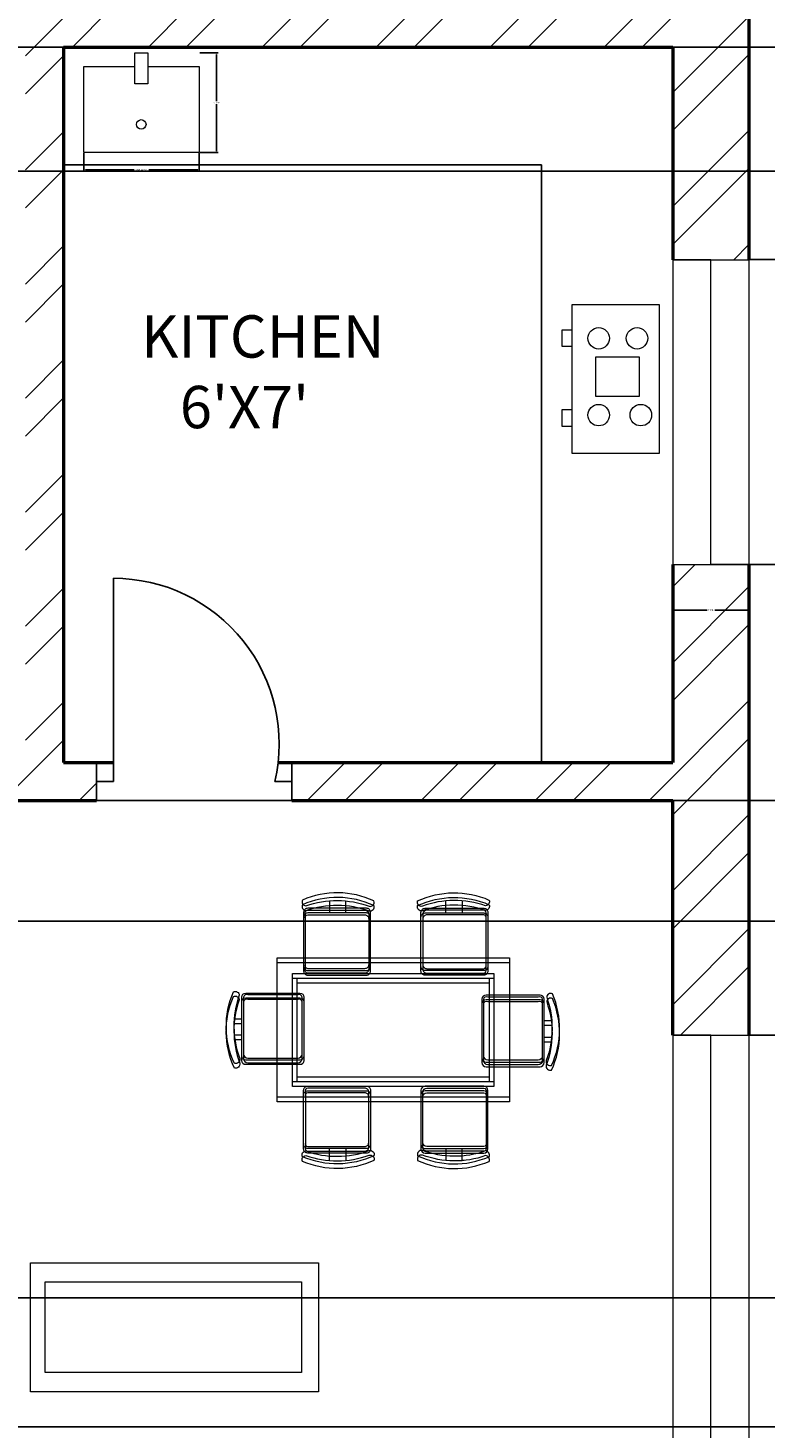
# Model space of a CAD drawing. Units: inches. Extents: x 2310 to 2937, y 1113 to 2410.
# Tile 21 of 23: x 2739 to 2826, y 2132 to 2297. Entities that reach past the tile are written whole.
import ezdxf

# ---------------------------------------------------------------- set-up
doc = ezdxf.new("R2010")
doc.units = ezdxf.units.IN
for name, color, linetype, lineweight in [('A-ANNO-DIMS', 2, 'Continuous', 18), ('A-AREA-IDEN', 7, 'Continuous', 18), ('A-DOOR', 31, 'Continuous', 25), ('A-EQPM', 8, 'Continuous', 18), ('A-FLOR-CASE', 7, 'Continuous', 25), ('A-FLOR-FIXT', 9, 'Continuous', 18), ('A-FURN', 8, 'Continuous', 18), ('A-GLAZ', 191, 'Continuous', 20), ('A-WALL', 7, 'Continuous', 50), ('A-WALL-PATT', 85, 'Continuous', 13)]:
    doc.layers.add(name, color=color, linetype=linetype, lineweight=lineweight)
doc.styles.get("Standard").update_dxf_attribs({"font": 'arial.ttf'})
doc.dimstyles.get("Standard").update_dxf_attribs({"dimtxt": 0.18, "dimasz": 0.18, "dimexe": 0.18, "dimexo": 0.0625, "dimgap": 0.09, "dimtad": 0, "dimtih": 1, "dimtoh": 1, "dimdec": 4, "dimzin": 0, "dimdsep": 46, "dimtxsty": 'Standard', "dimcen": 0.09, "dimadec": 0, "dimazin": 0, "dimtfac": 1, "dimtdec": 4, "dimtofl": 0, "dimtmove": 0, "dimatfit": 3, "dimfxl": 1, "dimtolj": 1, "dimtzin": 0, "dimarcsym": 0})

# ---------------------------------------------------------------- blocks, each defined once
blk = doc.blocks.new('SINK-KITCHEN')
blk.add_lwpolyline([(6.01, 11.79), (7.56, 11.79), (7.56, 8.11), (6.01, 8.11)], close=True)
blk.add_lwpolyline([(7.56, 10.17), (13.64, 10.17), (13.64, 0), (0, 0), (0, 10.17), (6.01, 10.17)])
blk.add_circle((6.79, 3.34), 0.556)
blk = doc.blocks.new('RANGE-4-BURNER')
for points in [[(1.2, 17.61), (1.2, 17.61), (1.2, 17.61), (1.2, 17.61)], [(1.2, 17.61), (11.5, 17.61), (11.5, 0), (1.2, 0)], [(1.2, 14.58), (0, 14.58), (0, 12.67), (1.2, 12.67)], [(4.01, 11.43), (9.13, 11.43), (9.13, 6.73), (4.01, 6.73)], [(1.2, 5.14), (0, 5.14), (0, 3.24), (1.2, 3.24)]]:
    blk.add_lwpolyline(points, close=True)
for centre in [(4.34, 13.6), (8.87, 13.6), (4.34, 4.53), (9.32, 4.53)]:
    blk.add_circle(centre, 1.27)
blk = doc.blocks.new('WIN-36IN')
for p, q in [((4.5, 36), (0, 36)), ((0, 36), (9, 36)), ((0, 36), (0, 0)), ((4.5, 0), (4.5, 36)), ((9, 36), (9, 0)), ((0, 0), (9, 0)), ((9, 0), (4.5, 0))]:
    blk.add_line(p, q)
blk = doc.blocks.new('DINING-TABLE')
for points in [[(0, 17.02), (27.45, 17.02), (27.45, 0.55), (0, 0.55)], [(0, 17.02), (27.45, 17.02), (27.45, 0.55), (0, 0.55)], [(0, 16.47), (27.45, 16.47), (27.45, 0), (0, 0)], [(0, 16.47), (27.45, 16.47), (27.45, 0), (0, 0)], [(1.83, 15.19), (25.62, 15.19), (25.62, 2.38), (1.83, 2.38)], [(1.83, 15.19), (25.62, 15.19), (25.62, 2.38), (1.83, 2.38)], [(1.83, 14.64), (25.62, 14.64), (25.62, 1.83), (1.83, 1.83)], [(1.83, 14.64), (25.62, 14.64), (25.62, 1.83), (1.83, 1.83)], [(2.38, 14.64), (25.07, 14.64), (25.07, 2.93), (2.38, 2.93)], [(2.38, 14.64), (25.07, 14.64), (25.07, 2.93), (2.38, 2.93)], [(2.38, 14.09), (25.07, 14.09), (25.07, 2.38), (2.38, 2.38)], [(2.38, 14.09), (25.07, 14.09), (25.07, 2.38), (2.38, 2.38)]]:
    blk.add_lwpolyline(points, close=True)
blk = doc.blocks.new('CHAIR-DINING')
for points in [[(0.62, 8.14, -0.578392), (0.05, 8.77, -0.214524), (8.49, 8.88, -0.552014), (8.09, 8.2, 0.175809), (0.62, 8.14)], [(0.62, 8.14, -0.578392), (0.05, 8.77, -0.214524), (8.49, 8.88, -0.552014), (8.09, 8.2, 0.175809), (0.62, 8.14)], [(0.62, 7.6, -0.578392), (0.05, 8.22, -0.214524), (8.49, 8.33, -0.552014), (8.09, 7.65, 0.175809), (0.62, 7.6)], [(0.62, 7.6, -0.578392), (0.05, 8.22, -0.214524), (8.49, 8.33, -0.552014), (8.09, 7.65, 0.175809), (0.62, 7.6)], [(3.37, 7.9), (3.37, 8.78, 0.064759)], [(3.37, 7.9), (3.37, 8.78, 0.064759)], [(7.88, 7.9, -0.414214), (8.36, 7.42), (8.36, 1.03, -0.414214), (7.88, 0.55), (0.94, 0.55, -0.414214), (0.45, 1.03), (0.45, 7.42, -0.414214), (0.94, 7.9), (7.88, 7.9)], [(7.88, 7.9, -0.414214), (8.36, 7.42), (8.36, 1.03, -0.414214), (7.88, 0.55), (0.94, 0.55, -0.414214), (0.45, 1.03), (0.45, 7.42, -0.414214), (0.94, 7.9), (7.88, 7.9)], [(7.88, 7.35, -0.414214), (8.36, 6.87), (8.36, 0.49, -0.414214), (7.88, 0), (0.94, 0, -0.414214), (0.45, 0.49), (0.45, 6.87, -0.414214), (0.94, 7.35), (7.88, 7.35)], [(7.88, 7.35, -0.414214), (8.36, 6.87), (8.36, 0.49, -0.414214), (7.88, 0), (0.94, 0, -0.414214), (0.45, 0.49), (0.45, 6.87, -0.414214), (0.94, 7.35), (7.88, 7.35)], [(3.37, 7.35), (3.37, 8.23, 0.064759)], [(3.37, 7.35), (3.37, 8.23, 0.064759)]]:
    blk.add_lwpolyline(points, format="xyb")
for points in [[(5.32, 8.8), (5.32, 7.9)], [(5.32, 8.79), (5.32, 7.9)], [(5.32, 8.25), (5.32, 7.35)], [(5.32, 8.25), (5.32, 7.35)]]:
    blk.add_lwpolyline(points)
for points in [[(7.87, 7.68), (1.16, 7.68, 0.414214), (0.67, 7.2), (0.67, 1.25, 0.414214), (1.16, 0.77), (7.87, 0.77, 0.512069), (8.14, 1.25), (8.14, 7.2, 0.512069)], [(7.87, 7.68), (1.16, 7.68, 0.414214), (0.67, 7.2), (0.67, 1.25, 0.414214), (1.16, 0.77), (7.87, 0.77, 0.512069), (8.14, 1.25), (8.14, 7.2, 0.512069)], [(7.87, 7.13), (1.16, 7.13, 0.414214), (0.67, 6.65), (0.67, 0.7, 0.414214), (1.16, 0.22), (7.87, 0.22, 0.512069), (8.14, 0.7), (8.14, 6.65, 0.512069)], [(7.87, 7.13), (1.16, 7.13, 0.414214), (0.67, 6.65), (0.67, 0.7, 0.414214), (1.16, 0.22), (7.87, 0.22, 0.512069), (8.14, 0.7), (8.14, 6.65, 0.512069)]]:
    blk.add_lwpolyline(points, format="xyb", close=True)
blk = doc.blocks.new('CHAIR-DINING-3')
for points in [[(0.47, 8.2, -0.175809), (7.95, 8.14, 0.578392), (8.51, 8.77, 0.214524), (0.07, 8.88, 0.552014), (0.47, 8.2, -0.065079)], [(0.47, 8.2, -0.175809), (7.95, 8.14, 0.578392), (8.51, 8.77, 0.214524), (0.07, 8.88, 0.552014), (0.47, 8.2, -0.065079)], [(0.47, 7.65, -0.175809), (7.95, 7.6, 0.578392), (8.51, 8.22, 0.214524), (0.07, 8.33, 0.552014), (0.47, 7.65, -0.065079)], [(0.47, 7.65, -0.175809), (7.95, 7.6, 0.578392), (8.51, 8.22, 0.214524), (0.07, 8.33, 0.552014), (0.47, 7.65, -0.065079)], [(5.19, 7.9), (5.19, 8.78, -0.064759)], [(5.19, 7.9), (5.19, 8.78, -0.064759)], [(7.63, 7.9), (0.69, 7.9, 0.414214), (0.2, 7.42), (0.2, 1.03, 0.414214), (0.69, 0.55), (7.63, 0.55, 0.414214), (8.11, 1.03), (8.11, 7.42, 0.414214), (7.63, 7.9)], [(7.63, 7.9), (0.69, 7.9, 0.414214), (0.2, 7.42), (0.2, 1.03, 0.414214), (0.69, 0.55), (7.63, 0.55, 0.414214), (8.11, 1.03), (8.11, 7.42, 0.414214), (7.63, 7.9)], [(7.63, 7.35), (0.69, 7.35, 0.414214), (0.2, 6.87), (0.2, 0.49, 0.414214), (0.69, 0), (7.63, 0, 0.414214), (8.11, 0.49), (8.11, 6.87, 0.414214), (7.63, 7.35)], [(7.63, 7.35), (0.69, 7.35, 0.414214), (0.2, 6.87), (0.2, 0.49, 0.414214), (0.69, 0), (7.63, 0, 0.414214), (8.11, 0.49), (8.11, 6.87, 0.414214), (7.63, 7.35)], [(5.19, 7.35), (5.19, 8.23, -0.064759)], [(5.19, 7.35), (5.19, 8.23, -0.064759)]]:
    blk.add_lwpolyline(points, format="xyb")
for points in [[(3.25, 8.8), (3.25, 7.9)], [(3.25, 8.79), (3.25, 7.9)], [(3.25, 8.25), (3.25, 7.35)], [(3.25, 8.25), (3.25, 7.35)]]:
    blk.add_lwpolyline(points)
for points in [[(0.69, 7.68), (7.41, 7.68, -0.414214), (7.9, 7.2), (7.9, 1.25, -0.414214), (7.41, 0.77), (0.69, 0.77, -0.512069), (0.42, 1.25), (0.42, 7.2, -0.512069)], [(0.69, 7.68), (7.41, 7.68, -0.414214), (7.9, 7.2), (7.9, 1.25, -0.414214), (7.41, 0.77), (0.69, 0.77, -0.512069), (0.42, 1.25), (0.42, 7.2, -0.512069)], [(0.69, 7.13), (7.41, 7.13, -0.414214), (7.9, 6.65), (7.9, 0.7, -0.414214), (7.41, 0.22), (0.69, 0.22, -0.512069), (0.42, 0.7), (0.42, 6.65, -0.512069)], [(0.69, 7.13), (7.41, 7.13, -0.414214), (7.9, 6.65), (7.9, 0.7, -0.414214), (7.41, 0.22), (0.69, 0.22, -0.512069), (0.42, 0.7), (0.42, 6.65, -0.512069)]]:
    blk.add_lwpolyline(points, format="xyb", close=True)
blk = doc.blocks.new('CHAIR-DINING-4')
for points in [[(0.62, 8.14, -0.578392), (0.05, 8.77, -0.214524), (8.49, 8.88, -0.552014), (8.09, 8.2, 0.175809), (0.62, 8.14)], [(0.62, 8.14, -0.578392), (0.05, 8.77, -0.214524), (8.49, 8.88, -0.552014), (8.09, 8.2, 0.175809), (0.62, 8.14)], [(0.62, 7.6, -0.578392), (0.05, 8.22, -0.214524), (8.49, 8.33, -0.552014), (8.09, 7.65, 0.175809), (0.62, 7.6)], [(0.62, 7.6, -0.578392), (0.05, 8.22, -0.214524), (8.49, 8.33, -0.552014), (8.09, 7.65, 0.175809), (0.62, 7.6)], [(3.37, 7.9), (3.37, 8.78, 0.064759)], [(3.37, 7.9), (3.37, 8.78, 0.064759)], [(7.88, 7.9, -0.414214), (8.36, 7.42), (8.36, 1.03, -0.414214), (7.88, 0.55), (0.94, 0.55, -0.414214), (0.45, 1.03), (0.45, 7.42, -0.414214), (0.94, 7.9), (7.88, 7.9)], [(7.88, 7.9, -0.414214), (8.36, 7.42), (8.36, 1.03, -0.414214), (7.88, 0.55), (0.94, 0.55, -0.414214), (0.45, 1.03), (0.45, 7.42, -0.414214), (0.94, 7.9), (7.88, 7.9)], [(7.88, 7.35, -0.414214), (8.36, 6.87), (8.36, 0.49, -0.414214), (7.88, 0), (0.94, 0, -0.414214), (0.45, 0.49), (0.45, 6.87, -0.414214), (0.94, 7.35), (7.88, 7.35)], [(7.88, 7.35, -0.414214), (8.36, 6.87), (8.36, 0.49, -0.414214), (7.88, 0), (0.94, 0, -0.414214), (0.45, 0.49), (0.45, 6.87, -0.414214), (0.94, 7.35), (7.88, 7.35)], [(3.37, 7.35), (3.37, 8.23, 0.064759)], [(3.37, 7.35), (3.37, 8.23, 0.064759)]]:
    blk.add_lwpolyline(points, format="xyb")
for points in [[(5.32, 8.8), (5.32, 7.9)], [(5.32, 8.79), (5.32, 7.9)], [(5.32, 8.25), (5.32, 7.35)], [(5.32, 8.25), (5.32, 7.35)]]:
    blk.add_lwpolyline(points)
for points in [[(7.87, 7.68), (1.16, 7.68, 0.414214), (0.67, 7.2), (0.67, 1.25, 0.414214), (1.16, 0.77), (7.87, 0.77, 0.512069), (8.14, 1.25), (8.14, 7.2, 0.512069)], [(7.87, 7.68), (1.16, 7.68, 0.414214), (0.67, 7.2), (0.67, 1.25, 0.414214), (1.16, 0.77), (7.87, 0.77, 0.512069), (8.14, 1.25), (8.14, 7.2, 0.512069)], [(7.87, 7.13), (1.16, 7.13, 0.414214), (0.67, 6.65), (0.67, 0.7, 0.414214), (1.16, 0.22), (7.87, 0.22, 0.512069), (8.14, 0.7), (8.14, 6.65, 0.512069)], [(7.87, 7.13), (1.16, 7.13, 0.414214), (0.67, 6.65), (0.67, 0.7, 0.414214), (1.16, 0.22), (7.87, 0.22, 0.512069), (8.14, 0.7), (8.14, 6.65, 0.512069)]]:
    blk.add_lwpolyline(points, format="xyb", close=True)
blk = doc.blocks.new('*D23')
at = {"layer": 'A-ANNO-DIMS', "color": 0, "lineweight": -2, "transparency": 16777216}
for p, q in [((2745.39, 2282.48), (2745.39, 2280.32)), ((2759.02, 2282.48), (2759.02, 2280.32)), ((2745.57, 2280.5), (2751.35, 2280.5)), ((2758.84, 2280.5), (2753.06, 2280.5))]:
    blk.add_line(p, q, dxfattribs=at)
at = {"layer": 'A-ANNO-DIMS', "color": 0, "transparency": 16777216}
for points in [[(2745.57, 2280.53), (2745.57, 2280.47), (2745.39, 2280.5)], [(2758.84, 2280.53), (2758.84, 2280.47), (2759.02, 2280.5)]]:
    blk.add_solid(points, dxfattribs=at)
at = {"layer": 'Defpoints', "color": 0, "transparency": 16777216}
for p in [(2745.39, 2282.54), (2759.02, 2282.54), (2759.02, 2280.5)]:
    blk.add_point(p, dxfattribs=at)
at = {"layer": 'A-ANNO-DIMS', "color": 0, "transparency": 16777216, "insert": (2752.2, 2280.5), "char_height": 0.18, "attachment_point": 5}
blk.add_mtext('\\A1;SINK 14 TYP.', dxfattribs=at)
blk = doc.blocks.new('*D24')
at = {"layer": 'A-ANNO-DIMS', "color": 0, "lineweight": -2, "transparency": 16777216}
for p, q in [((2759.09, 2294.33), (2761.25, 2294.33)), ((2761.07, 2294.15), (2761.07, 2288.62)), ((2761.07, 2282.72), (2761.07, 2288.26)), ((2759.09, 2282.54), (2761.25, 2282.54))]:
    blk.add_line(p, q, dxfattribs=at)
at = {"layer": 'A-ANNO-DIMS', "color": 0, "transparency": 16777216}
for points in [[(2761.04, 2294.15), (2761.1, 2294.15), (2761.07, 2294.33)], [(2761.04, 2282.72), (2761.1, 2282.72), (2761.07, 2282.54)]]:
    blk.add_solid(points, dxfattribs=at)
at = {"layer": 'Defpoints', "color": 0, "transparency": 16777216}
for p in [(2759.02, 2294.33), (2761.07, 2294.33), (2759.02, 2282.54)]:
    blk.add_point(p, dxfattribs=at)
at = {"layer": 'A-ANNO-DIMS', "color": 0, "transparency": 16777216, "insert": (2761.07, 2288.44), "char_height": 0.18, "attachment_point": 5}
blk.add_mtext('\\A1;12 TYP.', dxfattribs=at)
blk = doc.blocks.new('*D31')
at = {"layer": 'A-ANNO-DIMS', "color": 0, "lineweight": -2, "transparency": 16777216}
for p, q in [((2824.05, 2269.9), (2829.57, 2269.9)), ((2829.39, 2269.72), (2829.39, 2252.08)), ((2829.39, 2234.08), (2829.39, 2251.71)), ((2824.05, 2233.9), (2829.57, 2233.9))]:
    blk.add_line(p, q, dxfattribs=at)
at = {"layer": 'A-ANNO-DIMS', "color": 0, "transparency": 16777216}
for points in [[(2829.36, 2269.72), (2829.42, 2269.72), (2829.39, 2269.9)], [(2829.36, 2234.08), (2829.42, 2234.08), (2829.39, 2233.9)]]:
    blk.add_solid(points, dxfattribs=at)
at = {"layer": 'Defpoints', "color": 0, "transparency": 16777216}
for p in [(2823.99, 2269.9), (2829.39, 2269.9), (2823.99, 2233.9)]:
    blk.add_point(p, dxfattribs=at)
at = {"layer": 'A-ANNO-DIMS', "color": 0, "transparency": 16777216, "insert": (2829.39, 2251.9), "char_height": 0.18, "attachment_point": 5}
blk.add_mtext('\\A1;WINDOW 36 TYP.', dxfattribs=at)
blk = doc.blocks.new('*D32')
at = {"layer": 'A-ANNO-DIMS', "color": 0, "lineweight": -2, "transparency": 16777216}
for p, q in [((2814.99, 2233.84), (2814.99, 2228.32)), ((2823.99, 2233.84), (2823.99, 2228.32)), ((2815.17, 2228.5), (2819.03, 2228.5)), ((2823.81, 2228.5), (2819.94, 2228.5))]:
    blk.add_line(p, q, dxfattribs=at)
at = {"layer": 'A-ANNO-DIMS', "color": 0, "transparency": 16777216}
for points in [[(2815.17, 2228.53), (2815.17, 2228.47), (2814.99, 2228.5)], [(2823.81, 2228.53), (2823.81, 2228.47), (2823.99, 2228.5)]]:
    blk.add_solid(points, dxfattribs=at)
at = {"layer": 'Defpoints', "color": 0, "transparency": 16777216}
for p in [(2814.99, 2233.9), (2823.99, 2233.9), (2823.99, 2228.5)]:
    blk.add_point(p, dxfattribs=at)
at = {"layer": 'A-ANNO-DIMS', "color": 0, "transparency": 16777216, "insert": (2819.49, 2228.5), "char_height": 0.18, "attachment_point": 5}
blk.add_mtext('\\A1;9 TYP.', dxfattribs=at)
blk = doc.blocks.new('*D49')
at = {"layer": 'A-ANNO-DIMS', "color": 0, "lineweight": -2, "transparency": 16777216}
for p, q in [((2824.05, 2233.9), (2858.02, 2233.9)), ((2857.84, 2233.72), (2857.84, 2206.28)), ((2857.84, 2178.48), (2857.84, 2205.92)), ((2824.05, 2178.3), (2858.02, 2178.3))]:
    blk.add_line(p, q, dxfattribs=at)
at = {"layer": 'A-ANNO-DIMS', "color": 0, "transparency": 16777216}
for points in [[(2857.81, 2233.72), (2857.87, 2233.72), (2857.84, 2233.9)], [(2857.81, 2178.48), (2857.87, 2178.48), (2857.84, 2178.3)]]:
    blk.add_solid(points, dxfattribs=at)
at = {"layer": 'Defpoints', "color": 0, "transparency": 16777216}
for p in [(2823.99, 2233.9), (2857.84, 2233.9), (2823.99, 2178.3)]:
    blk.add_point(p, dxfattribs=at)
at = {"layer": 'A-ANNO-DIMS', "color": 0, "transparency": 16777216, "insert": (2857.84, 2206.1), "char_height": 0.18, "attachment_point": 5}
blk.add_mtext('\\A1;55.6', dxfattribs=at)
blk = doc.blocks.new('*D50')
at = {"layer": 'A-ANNO-DIMS', "color": 0, "lineweight": -2, "transparency": 16777216}
for p, q in [((2824.05, 2312.76), (2858.02, 2312.76)), ((2857.84, 2312.58), (2857.84, 2291.51)), ((2857.84, 2270.08), (2857.84, 2291.15)), ((2824.05, 2269.9), (2858.02, 2269.9))]:
    blk.add_line(p, q, dxfattribs=at)
at = {"layer": 'A-ANNO-DIMS', "color": 0, "transparency": 16777216}
for points in [[(2857.81, 2312.58), (2857.87, 2312.58), (2857.84, 2312.76)], [(2857.81, 2270.08), (2857.87, 2270.08), (2857.84, 2269.9)]]:
    blk.add_solid(points, dxfattribs=at)
at = {"layer": 'Defpoints', "color": 0, "transparency": 16777216}
for p in [(2823.99, 2312.76), (2857.84, 2312.76), (2823.99, 2269.9)]:
    blk.add_point(p, dxfattribs=at)
at = {"layer": 'A-ANNO-DIMS', "color": 0, "transparency": 16777216, "insert": (2857.84, 2291.33), "char_height": 0.18, "attachment_point": 5}
blk.add_mtext('\\A1;42.86', dxfattribs=at)
blk = doc.blocks.new('*D53')
at = {"layer": 'A-ANNO-DIMS', "color": 0, "lineweight": -2, "transparency": 16777216}
for p, q in [((2403.55, 2295.01), (2858.02, 2295.01)), ((2857.84, 2294.83), (2857.84, 2287.87)), ((2857.84, 2280.55), (2857.84, 2287.51)), ((2403.55, 2280.37), (2858.02, 2280.37))]:
    blk.add_line(p, q, dxfattribs=at)
at = {"layer": 'A-ANNO-DIMS', "color": 0, "transparency": 16777216}
for points in [[(2857.81, 2294.83), (2857.87, 2294.83), (2857.84, 2295.01)], [(2857.81, 2280.55), (2857.87, 2280.55), (2857.84, 2280.37)]]:
    blk.add_solid(points, dxfattribs=at)
at = {"layer": 'Defpoints', "color": 0, "transparency": 16777216}
for p in [(2403.49, 2295.01), (2403.49, 2280.37), (2857.84, 2280.37)]:
    blk.add_point(p, dxfattribs=at)
at = {"layer": 'A-ANNO-DIMS', "color": 0, "transparency": 16777216, "insert": (2857.84, 2287.69), "char_height": 0.18, "attachment_point": 5}
blk.add_mtext('\\A1;14.644', dxfattribs=at)
blk = doc.blocks.new('*D54')
at = {"layer": 'A-ANNO-DIMS', "color": 0, "lineweight": -2, "transparency": 16777216}
for p, q in [((2403.55, 2206.01), (2858.02, 2206.01)), ((2857.84, 2205.83), (2857.84, 2199.07)), ((2857.84, 2191.94), (2857.84, 2198.7)), ((2403.55, 2191.76), (2858.02, 2191.76))]:
    blk.add_line(p, q, dxfattribs=at)
at = {"layer": 'A-ANNO-DIMS', "color": 0, "transparency": 16777216}
for points in [[(2857.81, 2205.83), (2857.87, 2205.83), (2857.84, 2206.01)], [(2857.81, 2191.94), (2857.87, 2191.94), (2857.84, 2191.76)]]:
    blk.add_solid(points, dxfattribs=at)
at = {"layer": 'Defpoints', "color": 0, "transparency": 16777216}
for p in [(2403.49, 2206.01), (2403.49, 2191.76), (2857.84, 2191.76)]:
    blk.add_point(p, dxfattribs=at)
at = {"layer": 'A-ANNO-DIMS', "color": 0, "transparency": 16777216, "insert": (2857.84, 2198.89), "char_height": 0.18, "attachment_point": 5}
blk.add_mtext('\\A1;14.255', dxfattribs=at)
blk = doc.blocks.new('*D70')
at = {"layer": 'A-ANNO-DIMS', "color": 0, "lineweight": -2, "transparency": 16777216}
for p, q in [((2475.96, 2147.28), (2858.02, 2147.28)), ((2857.84, 2147.1), (2857.84, 2139.83)), ((2857.84, 2132.2), (2857.84, 2139.47)), ((2475.96, 2132.02), (2858.02, 2132.02))]:
    blk.add_line(p, q, dxfattribs=at)
at = {"layer": 'A-ANNO-DIMS', "color": 0, "transparency": 16777216}
for points in [[(2857.81, 2147.1), (2857.87, 2147.1), (2857.84, 2147.28)], [(2857.81, 2132.2), (2857.87, 2132.2), (2857.84, 2132.02)]]:
    blk.add_solid(points, dxfattribs=at)
at = {"layer": 'Defpoints', "color": 0, "transparency": 16777216}
for p in [(2475.89, 2147.28), (2857.84, 2147.28), (2475.89, 2132.02)]:
    blk.add_point(p, dxfattribs=at)
at = {"layer": 'A-ANNO-DIMS', "color": 0, "transparency": 16777216, "insert": (2857.84, 2139.65), "char_height": 0.18, "attachment_point": 5}
blk.add_mtext('\\A1;15.257', dxfattribs=at)

msp = doc.modelspace()

# ---------------------------------------------------------------- hatches: boundary and pattern name
at = {"layer": 'A-WALL-PATT'}
h = msp.add_hatch(dxfattribs=at)
h.set_pattern_fill('ANSI32', color=256)
h.paths.add_polyline_path([(2639.1394, 2356.5139), (2563.662, 2356.5139), (2563.662, 2347.5139), (2606.9859, 2347.5139), (2606.9859, 2210.5139), (2514.2692, 2210.5139), (2514.2692, 2206.0139), (2606.9859, 2206.0139), (2606.9859, 2098.0139), (2602.689, 2098.0139), (2602.689, 2093.5139), (2615.5262, 2093.5139), (2615.5262, 2095.7639), (2615.5262, 2098.0139), (2611.4859, 2098.0139), (2611.4859, 2206.0139), (2703.9391, 2206.0139), (2703.9391, 2208.2639), (2703.9391, 2210.5139), (2611.4859, 2210.5139), (2611.4859, 2347.5139), (2639.1394, 2347.5139)])
h.paths.add_polyline_path([(2823.9859, 2356.5139), (2699.1394, 2356.5139), (2699.1394, 2347.5139), (2738.4859, 2347.5139), (2738.4859, 2343.9266), (2742.9859, 2343.9266), (2742.9859, 2347.5139), (2814.9859, 2347.5139), (2814.9859, 2336.76), (2823.9859, 2336.76)])
h.paths.add_polyline_path([(2823.9859, 2312.76), (2814.9859, 2312.76), (2814.9859, 2299.5139), (2742.9859, 2299.5139), (2742.9859, 2323.0159), (2740.7359, 2323.0159), (2738.4859, 2323.0159), (2738.4859, 2210.5139), (2734.5483, 2210.5139), (2734.5483, 2206.0139), (2746.8769, 2206.0139), (2746.8769, 2208.2639), (2746.8769, 2210.5139), (2742.9859, 2210.5139), (2742.9859, 2295.0139), (2814.9859, 2295.0139), (2814.9859, 2269.8977), (2823.9859, 2269.8977)])
h.paths.add_polyline_path([(2823.9859, 2210.5139), (2823.9859, 2233.8977), (2819.4859, 2233.8977), (2814.9859, 2233.8977), (2814.9859, 2210.5139), (2769.9745, 2210.5139), (2769.9745, 2206.0139), (2814.9859, 2206.0139), (2814.9859, 2178.3027), (2823.9859, 2178.3027)])
h.paths.add_polyline_path([(2823.9859, 2118.3027), (2819.4859, 2118.3027), (2814.9859, 2118.3027), (2814.9859, 2098.0139), (2647.0333, 2098.0139), (2647.0333, 2093.5139), (2814.9859, 2093.5139), (2814.9859, 1999.5139), (2650.6052, 1999.5139), (2650.6052, 1995.0139), (2814.9859, 1995.0139), (2814.9859, 1969.9784), (2823.9859, 1969.9784)])
h.paths.add_polyline_path([(2403.4859, 2093.5139), (2569.9888, 2093.5139), (2569.9888, 2095.7639), (2569.9888, 2098.0139), (2403.4859, 2098.0139), (2403.4859, 2131.7587), (2394.4859, 2131.7587), (2394.4859, 1967.522), (2403.4859, 1967.522), (2403.4859, 1995.0139), (2569.8903, 1995.0139), (2569.8903, 1997.2639), (2569.8903, 1999.5139), (2403.4859, 1999.5139)])
h.paths.add_polyline_path([(2503.662, 2356.5139), (2394.4859, 2356.5139), (2394.4859, 2337.9231), (2398.9859, 2337.9231), (2403.4859, 2337.9231), (2403.4859, 2347.5139), (2475.4859, 2347.5139), (2475.4859, 2343.0384), (2479.9859, 2343.0384), (2479.9859, 2347.5139), (2503.662, 2347.5139)])
h.paths.add_polyline_path([(2498.3065, 1745.5139), (2479.9859, 1745.5139), (2479.9859, 1749.1663), (2477.7359, 1749.1663), (2475.4859, 1749.1663), (2475.4859, 1745.5139), (2403.4859, 1745.5139), (2403.4859, 1753.6409), (2398.9859, 1753.6409), (2394.4859, 1753.6409), (2394.4859, 1736.5139), (2498.3065, 1736.5139), (2498.3065, 1741.0139)])
h.paths.add_polyline_path([(2479.9859, 1882.5139), (2483.9367, 1882.5139), (2483.9367, 1887.0139), (2471.5501, 1887.0139), (2471.5501, 1885.1969), (2471.5501, 1882.5139), (2475.4859, 1882.5139), (2475.4859, 1798.0139), (2403.4859, 1798.0139), (2403.4859, 1828.0433), (2402.2852, 1828.0433), (2394.4859, 1828.0433), (2394.4859, 1777.6409), (2403.4859, 1777.6409), (2403.4859, 1793.5139), (2475.4859, 1793.5139), (2475.4859, 1769.1696), (2479.9859, 1769.1696)])
h.paths.add_polyline_path([(2403.4859, 1907.522), (2398.9859, 1907.522), (2394.4859, 1907.522), (2394.4859, 1864.0433), (2403.4859, 1864.0433), (2403.4859, 1882.5139), (2448.9325, 1882.5139), (2448.9325, 1884.7639), (2448.9325, 1887.0139), (2403.4859, 1887.0139)])
h.paths.add_polyline_path([(2702.2061, 1887.0139), (2611.4859, 1887.0139), (2611.4859, 1995.0139), (2615.6132, 1995.0139), (2615.6132, 1999.5139), (2602.4798, 1999.5139), (2602.4798, 1997.2639), (2602.4798, 1995.0139), (2606.9859, 1995.0139), (2606.9859, 1887.0139), (2516.2443, 1887.0139), (2516.2443, 1884.7639), (2516.2443, 1882.5139), (2606.9859, 1882.5139), (2606.9859, 1745.5139), (2558.3065, 1745.5139), (2558.3065, 1736.5139), (2638.8921, 1736.5139), (2638.8921, 1741.0139), (2638.8921, 1745.5139), (2611.4859, 1745.5139), (2611.4859, 1882.5139), (2702.2061, 1882.5139)])
h.paths.add_polyline_path([(2823.9859, 1909.9784), (2819.4859, 1909.9784), (2814.9859, 1909.9784), (2814.9859, 1887.0139), (2769.144, 1887.0139), (2769.144, 1884.7639), (2769.144, 1882.5139), (2814.9859, 1882.5139), (2814.9859, 1854.1704), (2823.9859, 1854.1704)])
h.paths.add_polyline_path([(2823.9859, 1818.1704), (2819.4859, 1818.1704), (2814.9859, 1818.1704), (2814.9859, 1798.0139), (2742.9859, 1798.0139), (2742.9859, 1882.5139), (2746.805, 1882.5139), (2746.805, 1887.0139), (2733.7334, 1887.0139), (2733.7334, 1884.7639), (2733.7334, 1882.5139), (2738.4859, 1882.5139), (2738.4859, 1771.1728), (2740.7359, 1771.1728), (2742.9859, 1771.1728), (2742.9859, 1793.5139), (2814.9859, 1793.5139), (2814.9859, 1783.6684), (2823.9859, 1783.6684)])
h.paths.add_polyline_path([(2823.9859, 1759.6684), (2814.9859, 1759.6684), (2814.9859, 1745.5139), (2742.9859, 1745.5139), (2742.9859, 1748.9831), (2740.7359, 1748.9831), (2738.4859, 1748.9831), (2738.4859, 1745.5139), (2698.8921, 1745.5139), (2698.8921, 1736.5139), (2823.9859, 1736.5139)])

# ---------------------------------------------------------------- linework, layer by layer
at = {"layer": 'A-DOOR'}
for p, q in [((2748.8769, 2208.2639), (2748.8769, 2232.2639)), ((2746.8769, 2210.5139), (2746.8769, 2210.5139)), ((2746.8769, 2210.5139), (2746.8769, 2206.0139)), ((2769.9745, 2210.5139), (2769.9745, 2206.0139)), ((2746.8769, 2206.0139), (2746.8769, 2208.2639)), ((2746.8769, 2208.2639), (2748.8769, 2208.2639)), ((2769.9745, 2208.2639), (2767.9745, 2208.2639)), ((2769.9745, 2206.0139), (2769.9745, 2208.2639))]:
    msp.add_line(p, q, dxfattribs=at)
msp.add_arc((2748.8769, 2212.6656), 19.5983, 347.020924, 90, dxfattribs=at)
at = {"layer": 'A-FLOR-CASE'}
for p, q in [((2799.45, 2281.1), (2742.9859, 2281.1)), ((2799.45, 2210.5139), (2799.45, 2281.1))]:
    msp.add_line(p, q, dxfattribs=at)
at = {"layer": 'A-FURN'}
for points in [[(2763.8047, 2175.5296, -0.57839206), (2763.182, 2174.9633, -0.21452438), (2763.0688, 2183.4015, -0.55201397), (2763.7481, 2183.005, 0.17580937), (2763.8047, 2175.5296)], [(2763.8048, 2175.5293, -0.57839206), (2763.182, 2174.963, -0.21452438), (2763.0688, 2183.4012, -0.55201397), (2763.7481, 2183.0048, 0.17580937), (2763.8048, 2175.5293)], [(2763.8047, 2174.9807, -0.57839206), (2763.182, 2174.4144, -0.21452438), (2763.0688, 2182.8526, -0.55201397), (2763.7481, 2182.4561, 0.17580937), (2763.8047, 2174.9807)], [(2763.8048, 2174.9804, -0.57839206), (2763.182, 2174.4141, -0.21452438), (2763.0688, 2182.8523, -0.55201397), (2763.7481, 2182.4558, 0.17580937), (2763.8048, 2174.9804)], [(2764.0482, 2182.7867, -0.41421356), (2764.5337, 2183.2722), (2770.9148, 2183.2722, -0.41421356), (2771.4004, 2182.7867), (2771.4004, 2175.8468, -0.41421356), (2770.9148, 2175.3612), (2764.5337, 2175.3612, -0.41421356), (2764.0482, 2175.8468), (2764.0482, 2182.7867)], [(2764.0482, 2182.7864, -0.41421356), (2764.5337, 2183.2719), (2770.9148, 2183.2719, -0.41421356), (2771.4004, 2182.7864), (2771.4004, 2175.8465, -0.41421356), (2770.9148, 2175.3609), (2764.5337, 2175.3609, -0.41421356), (2764.0482, 2175.8465), (2764.0482, 2182.7864)], [(2799.7856, 2182.549, 0.41421356), (2799.3001, 2183.0346), (2792.9189, 2183.0346, 0.41421356), (2792.4334, 2182.549), (2792.4334, 2175.6091, 0.41421356), (2792.9189, 2175.1236), (2799.3001, 2175.1236, 0.41421356), (2799.7856, 2175.6091), (2799.7856, 2182.549)], [(2799.7856, 2182.5487, 0.41421356), (2799.3001, 2183.0343), (2792.919, 2183.0343, 0.41421356), (2792.4334, 2182.5487), (2792.4334, 2175.6088, 0.41421356), (2792.919, 2175.1233), (2799.3001, 2175.1233, 0.41421356), (2799.7856, 2175.6088), (2799.7856, 2182.5487)], [(2800.0856, 2182.7674, -0.17580919), (2800.029, 2175.2919, 0.57839206), (2800.6518, 2174.7256, 0.21452438), (2800.765, 2183.1638, 0.55201397), (2800.0856, 2182.7674, -0.06507904)], [(2800.0857, 2182.7671, -0.17580919), (2800.0291, 2175.2916, 0.57839206), (2800.6518, 2174.7253, 0.21452438), (2800.765, 2183.1635, 0.55201397), (2800.0857, 2182.7671, -0.06507904)], [(2764.0482, 2182.2378, -0.41421356), (2764.5337, 2182.7233), (2770.9148, 2182.7233, -0.41421356), (2771.4004, 2182.2378), (2771.4004, 2175.2978, -0.41421356), (2770.9148, 2174.8123), (2764.5337, 2174.8123, -0.41421356), (2764.0482, 2175.2978), (2764.0482, 2182.2378)], [(2764.0482, 2182.2375, -0.41421356), (2764.5337, 2182.723), (2770.9148, 2182.723, -0.41421356), (2771.4004, 2182.2375), (2771.4004, 2175.2976, -0.41421356), (2770.9148, 2174.812), (2764.5337, 2174.812, -0.41421356), (2764.0482, 2175.2976), (2764.0482, 2182.2375)], [(2799.7856, 2182.0001, 0.41421356), (2799.3001, 2182.4856), (2792.9189, 2182.4856, 0.41421356), (2792.4334, 2182.0001), (2792.4334, 2175.0602, 0.41421356), (2792.9189, 2174.5746), (2799.3001, 2174.5746, 0.41421356), (2799.7856, 2175.0602), (2799.7856, 2182.0001)], [(2799.7856, 2181.9998, 0.41421356), (2799.3001, 2182.4853), (2792.919, 2182.4853, 0.41421356), (2792.4334, 2181.9998), (2792.4334, 2175.0599, 0.41421356), (2792.919, 2174.5744), (2799.3001, 2174.5744, 0.41421356), (2799.7856, 2175.0599), (2799.7856, 2181.9998)], [(2800.0856, 2182.2185, -0.17580919), (2800.029, 2174.743, 0.57839206), (2800.6518, 2174.1767, 0.21452438), (2800.765, 2182.6149, 0.55201397), (2800.0856, 2182.2185, -0.06507904)], [(2800.0857, 2182.2182, -0.17580919), (2800.0291, 2174.7427, 0.57839206), (2800.6518, 2174.1764, 0.21452438), (2800.765, 2182.6146, 0.55201397), (2800.0857, 2182.2182, -0.06507904)], [(2764.0482, 2178.2844), (2763.1705, 2178.2844, 0.06475861)], [(2764.0482, 2178.2841), (2763.1705, 2178.2841, 0.06475861)], [(2799.7856, 2178.0467), (2800.6633, 2178.0467, -0.06475861)], [(2799.7856, 2178.0465), (2800.6633, 2178.0465, -0.06475861)], [(2764.0482, 2177.7355), (2763.1705, 2177.7355, 0.06475861)], [(2764.0482, 2177.7352), (2763.1705, 2177.7352, 0.06475861)], [(2799.7856, 2177.4978), (2800.6633, 2177.4978, -0.06475861)], [(2799.7856, 2177.4975), (2800.6633, 2177.4975, -0.06475861)], [(2792.6514, 2164.9159, 0.41421356), (2793.1369, 2165.4014), (2793.1369, 2171.7826, 0.41421356), (2792.6514, 2172.2681), (2785.7114, 2172.2681, 0.41421356), (2785.2259, 2171.7826), (2785.2259, 2165.4014, 0.41421356), (2785.7114, 2164.9159), (2792.6514, 2164.9159)], [(2792.6514, 2164.9156, 0.41421356), (2793.1369, 2165.4011), (2793.1369, 2171.7823, 0.41421356), (2792.6514, 2172.2678), (2785.7114, 2172.2678, 0.41421356), (2785.2259, 2171.7823), (2785.2259, 2165.4011, 0.41421356), (2785.7114, 2164.9156), (2792.6514, 2164.9156)], [(2792.6514, 2164.367, 0.41421356), (2793.1369, 2164.8525), (2793.1369, 2171.2336, 0.41421356), (2792.6514, 2171.7192), (2785.7114, 2171.7192, 0.41421356), (2785.2259, 2171.2336), (2785.2259, 2164.8525, 0.41421356), (2785.7114, 2164.367), (2792.6514, 2164.367)], [(2792.6514, 2164.3667, 0.41421356), (2793.1369, 2164.8522), (2793.1369, 2171.2333, 0.41421356), (2792.6514, 2171.7189), (2785.7114, 2171.7189, 0.41421356), (2785.2259, 2171.2333), (2785.2259, 2164.8522, 0.41421356), (2785.7114, 2164.3667), (2792.6514, 2164.3667)], [(2788.1491, 2164.9159), (2788.1491, 2164.0382, -0.06475861)], [(2788.1491, 2164.9156), (2788.1491, 2164.0379, -0.06475861)], [(2792.8697, 2164.6159, -0.17580928), (2785.3943, 2164.6725, 0.57839206), (2784.828, 2164.0497, 0.21452438), (2793.2661, 2163.9365, 0.55201397), (2792.8697, 2164.6159, -0.06507904)], [(2792.8697, 2164.6156, -0.17580928), (2785.3943, 2164.6722, 0.57839206), (2784.828, 2164.0495, 0.21452438), (2793.2662, 2163.9362, 0.55201397), (2792.8697, 2164.6156, -0.06507904)], [(2792.8697, 2164.0669, -0.17580928), (2785.3943, 2164.1235, 0.57839206), (2784.828, 2163.5008, 0.21452438), (2793.2661, 2163.3876, 0.55201397), (2792.8697, 2164.0669, -0.06507904)], [(2792.8697, 2164.0666, -0.17580928), (2785.3943, 2164.1233, 0.57839206), (2784.828, 2163.5005, 0.21452438), (2793.2662, 2163.3873, 0.55201397), (2792.8697, 2164.0666, -0.06507904)], [(2788.1491, 2164.367), (2788.1491, 2163.4893, -0.06475861)], [(2788.1491, 2164.3667), (2788.1491, 2163.489, -0.06475861)]]:
    msp.add_lwpolyline(points, format="xyb", dxfattribs=at)
for points in [[(2764.2669, 2182.7838), (2764.2669, 2176.0655, 0.41421356), (2764.7524, 2175.58), (2770.6961, 2175.58, 0.41421356), (2771.1816, 2176.0655), (2771.1816, 2182.7838, 0.51206948), (2770.6961, 2183.0535), (2764.7524, 2183.0535, 0.51206948)], [(2764.2669, 2182.7835), (2764.2669, 2176.0652, 0.41421356), (2764.7524, 2175.5797), (2770.6961, 2175.5797, 0.41421356), (2771.1816, 2176.0652), (2771.1816, 2182.7835, 0.51206948), (2770.6961, 2183.0532), (2764.7524, 2183.0532, 0.51206948)], [(2764.2669, 2182.2348), (2764.2669, 2175.5166, 0.41421356), (2764.7524, 2175.0311), (2770.6961, 2175.0311, 0.41421356), (2771.1816, 2175.5166), (2771.1816, 2182.2348, 0.51206948), (2770.6961, 2182.5046), (2764.7524, 2182.5046, 0.51206948)], [(2764.2669, 2182.2346), (2764.2669, 2175.5163, 0.41421356), (2764.7524, 2175.0308), (2770.6961, 2175.0308, 0.41421356), (2771.1816, 2175.5163), (2771.1816, 2182.2346, 0.51206948), (2770.6961, 2182.5043), (2764.7524, 2182.5043, 0.51206948)], [(2799.5669, 2182.5461), (2799.5669, 2175.8278, -0.41421356), (2799.0814, 2175.3423), (2793.1377, 2175.3423, -0.41421356), (2792.6522, 2175.8278), (2792.6522, 2182.5461, -0.51206948), (2793.1377, 2182.8158), (2799.0814, 2182.8158, -0.51206948)], [(2799.5669, 2182.5458), (2799.5669, 2175.8275, -0.41421356), (2799.0814, 2175.342), (2793.1377, 2175.342, -0.41421356), (2792.6522, 2175.8275), (2792.6522, 2182.5458, -0.51206948), (2793.1377, 2182.8155), (2799.0814, 2182.8155, -0.51206948)], [(2799.5669, 2181.9972), (2799.5669, 2175.2789, -0.41421356), (2799.0814, 2174.7934), (2793.1377, 2174.7934, -0.41421356), (2792.6522, 2175.2789), (2792.6522, 2181.9972, -0.51206948), (2793.1377, 2182.2669), (2799.0814, 2182.2669, -0.51206948)], [(2799.5669, 2181.9969), (2799.5669, 2175.2786, -0.41421356), (2799.0814, 2174.7931), (2793.1377, 2174.7931, -0.41421356), (2792.6522, 2175.2786), (2792.6522, 2181.9969, -0.51206948), (2793.1377, 2182.2666), (2799.0814, 2182.2666, -0.51206948)], [(2792.6484, 2165.1346), (2785.9302, 2165.1346, -0.41421356), (2785.4446, 2165.6201), (2785.4446, 2171.5638, -0.41421356), (2785.9302, 2172.0493), (2792.6484, 2172.0493, -0.51206948), (2792.9182, 2171.5638), (2792.9182, 2165.6201, -0.51206948)], [(2792.6484, 2165.1343), (2785.9302, 2165.1343, -0.41421356), (2785.4446, 2165.6199), (2785.4446, 2171.5635, -0.41421356), (2785.9302, 2172.0491), (2792.6484, 2172.0491, -0.51206948), (2792.9182, 2171.5635), (2792.9182, 2165.6199, -0.51206948)], [(2792.6484, 2164.5857), (2785.9302, 2164.5857, -0.41421356), (2785.4446, 2165.0712), (2785.4446, 2171.0149, -0.41421356), (2785.9302, 2171.5004), (2792.6484, 2171.5004, -0.51206948), (2792.9182, 2171.0149), (2792.9182, 2165.0712, -0.51206948)], [(2792.6484, 2164.5854), (2785.9302, 2164.5854, -0.41421356), (2785.4446, 2165.0709), (2785.4446, 2171.0146, -0.41421356), (2785.9302, 2171.5001), (2792.6484, 2171.5001, -0.51206948), (2792.9182, 2171.0146), (2792.9182, 2165.0709, -0.51206948)]]:
    msp.add_lwpolyline(points, format="xyb", close=True, dxfattribs=at)
for points in [[(2763.1545, 2180.227), (2764.0482, 2180.227)], [(2763.1545, 2180.2267), (2764.0482, 2180.2267)], [(2763.1545, 2179.6781), (2764.0482, 2179.6781)], [(2763.1545, 2179.6778), (2764.0482, 2179.6778)], [(2800.6793, 2179.9893), (2799.7856, 2179.9893)], [(2800.6793, 2179.989), (2799.7856, 2179.989)], [(2800.6793, 2179.4404), (2799.7856, 2179.4404)], [(2800.6793, 2179.4401), (2799.7856, 2179.4401)], [(2790.0917, 2164.0222), (2790.0917, 2164.9159)], [(2790.0917, 2164.022), (2790.0917, 2164.9156)], [(2790.0917, 2163.4733), (2790.0917, 2164.367)], [(2790.0917, 2163.473), (2790.0917, 2164.3667)]]:
    msp.add_lwpolyline(points, dxfattribs=at)
for points in [[(2739.0835, 2151.4159), (2773.1151, 2151.4159), (2773.1151, 2136.1585), (2739.0835, 2136.1585)], [(2740.8089, 2149.1503), (2771.1145, 2149.1503), (2771.1145, 2138.4687), (2740.8089, 2138.4687)]]:
    msp.add_lwpolyline(points, close=True, dxfattribs=at)
at = {"layer": 'A-GLAZ'}
for p, q in [((2814.9859, 2269.8977), (2814.9859, 2269.8977)), ((2814.9859, 2269.8977), (2814.9859, 2269.8977)), ((2819.4859, 2178.3027), (2814.9859, 2178.3027)), ((2814.9859, 2178.3027), (2823.9859, 2178.3027)), ((2814.9859, 2178.3027), (2814.9859, 2118.3027)), ((2819.4859, 2118.3027), (2819.4859, 2178.3027)), ((2823.9859, 2178.3027), (2823.9859, 2118.0952))]:
    msp.add_line(p, q, dxfattribs=at)
at = {"layer": 'A-WALL'}
for p, q in [((2823.9859, 2312.76), (2823.9859, 2269.8977)), ((2742.9859, 2295.0139), (2814.9859, 2295.0139)), ((2742.9859, 2295.0139), (2742.9859, 2210.5139)), ((2814.9859, 2295.0139), (2814.9859, 2269.8977)), ((2814.9859, 2233.8977), (2814.9859, 2210.5139)), ((2823.9859, 2233.8977), (2823.9859, 2210.5139)), ((2742.9859, 2210.5139), (2748.8769, 2210.5139)), ((2768.3567, 2210.5139), (2814.9859, 2210.5139)), ((2823.9859, 2210.5139), (2823.9859, 2178.3027)), ((2734.5483, 2206.0139), (2746.8769, 2206.0139)), ((2769.9745, 2206.0139), (2814.9859, 2206.0139)), ((2814.9859, 2178.3027), (2814.9859, 2206.0139))]:
    msp.add_line(p, q, dxfattribs=at)

# ---------------------------------------------------------------- block references
at = {"layer": 'A-EQPM'}
msp.add_blockref('RANGE-4-BURNER', (2801.8879, 2247.0096), dxfattribs=at)
at = {"layer": 'A-FLOR-FIXT'}
msp.add_blockref('SINK-KITCHEN', (2745.3862, 2282.5424), dxfattribs=at)
at = {"layer": 'A-FURN'}
for name, p in [('CHAIR-DINING-3', (2771.1552, 2185.3802)), ('CHAIR-DINING-4', (2784.7748, 2185.3802)), ('DINING-TABLE', (2768.2307, 2170.404))]:
    msp.add_blockref(name, p, dxfattribs=at)
at = {"layer": 'A-FURN', "rotation": 180}
msp.add_blockref('CHAIR-DINING', (2779.7204, 2172.2681), dxfattribs=at)
at = {"layer": 'A-GLAZ'}
msp.add_blockref('WIN-36IN', (2814.9859, 2233.8977), dxfattribs=at)

# ---------------------------------------------------------------- texts
at = {"layer": 'A-AREA-IDEN', "insert": (2742.9859, 2263.3281), "char_height": 5, "attachment_point": 1}
msp.add_mtext_dynamic_manual_height_columns("      KITCHEN\\P         6'X7'", width=82.419571, gutter_width=12.5, heights=[0], dxfattribs=at)

# ---------------------------------------------------------------- dimensions: what is measured, and where the dimension line sits
at = {"layer": 'A-ANNO-DIMS'}
for base, p1, p2, override, picture, middle in [((2857.8359, 2312.76), (2823.9859, 2269.8977), (2823.9859, 2312.76), {"dimdec": 2, "dimlfac": 1, "dimrnd": 0, "dimzin": 0, "dimdsep": 46, "dimlunit": 2}, '*D50', (2857.8359, 2291.3288)), ((2857.8359, 2280.3697), (2403.4859, 2295.0139), (2403.4859, 2280.3697), {"dimdec": 3, "dimlfac": 1, "dimrnd": 0, "dimzin": 0, "dimdsep": 46, "dimlunit": 2}, '*D53', (2857.8359, 2287.6918)), ((2857.8359, 2233.8977), (2823.9859, 2178.3027), (2823.9859, 2233.8977), {"dimdec": 1, "dimlfac": 1, "dimrnd": 0, "dimzin": 0, "dimdsep": 46, "dimlunit": 2}, '*D49', (2857.8359, 2206.1002)), ((2857.8359, 2191.7587), (2403.4859, 2206.0139), (2403.4859, 2191.7587), {"dimdec": 3, "dimlfac": 1, "dimrnd": 0, "dimzin": 0, "dimdsep": 46, "dimlunit": 2}, '*D54', (2857.8359, 2198.8863)), ((2857.8359, 2147.2815), (2475.8929, 2132.0241), (2475.8929, 2147.2815), {"dimdec": 3, "dimlfac": 1, "dimrnd": 0, "dimzin": 0, "dimdsep": 46, "dimlunit": 2}, '*D70', (2857.8359, 2139.6528))]:
    dim = msp.add_linear_dim(base=base, p1=p1, p2=p2, angle=90, dimstyle='Standard', override=override, dxfattribs=at)
    dim.commit()
    dim.dimension.update_dxf_attribs({"geometry": picture, "text_midpoint": middle})
for base, p1, p2, text, picture, middle in [((2761.0686, 2294.3347), (2759.023, 2282.5424), (2759.023, 2294.3347), '<> TYP.', '*D24', (2761.0686, 2288.4386)), ((2829.3859, 2269.8977), (2823.9859, 2233.8977), (2823.9859, 2269.8977), 'WINDOW <> TYP.', '*D31', (2829.3859, 2251.8977))]:
    dim = msp.add_linear_dim(base=base, p1=p1, p2=p2, angle=90, text=text, dimstyle='Standard', override={"dimdec": 0, "dimlfac": 1, "dimrnd": 0, "dimzin": 0, "dimdsep": 46, "dimlunit": 2}, dxfattribs=at)
    dim.commit()
    dim.dimension.update_dxf_attribs({"geometry": picture, "text_midpoint": middle})
for base, p1, p2, text, picture, middle in [((2759.023, 2280.4969), (2745.3862, 2282.5424), (2759.023, 2282.5424), 'SINK <> TYP.', '*D23', (2752.2046, 2280.4969)), ((2823.9859, 2228.4977), (2814.9859, 2233.8977), (2823.9859, 2233.8977), '<> TYP.', '*D32', (2819.4859, 2228.4977))]:
    dim = msp.add_linear_dim(base=base, p1=p1, p2=p2, text=text, dimstyle='Standard', override={"dimdec": 0, "dimlfac": 1, "dimrnd": 0, "dimzin": 0, "dimdsep": 46, "dimlunit": 2}, dxfattribs=at)
    dim.commit()
    dim.dimension.update_dxf_attribs({"geometry": picture, "text_midpoint": middle})

doc.saveas('drawing.dxf')
